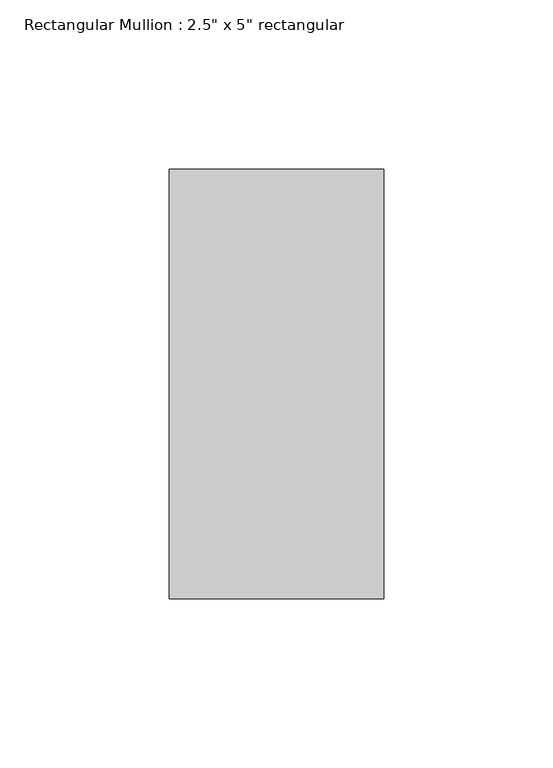
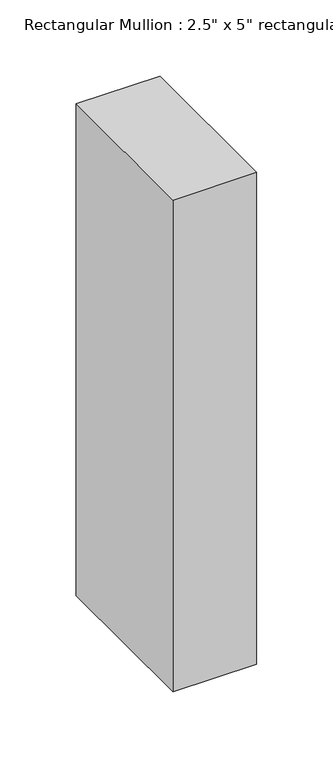
"""IFC4 building model written with IfcOpenShell, lengths in millimetres: member geometry."""

from ifc_helpers import new_model, si_unit, frame, origin, place, context, project, spatial, polyline, outline, extrude, source, transform, mapped, element, save


def member_7096a90e(model_context):
    return source(origin(), model_context, "Body", "SweptSolid", [
        extrude(outline(polyline([(0.0, 63.5), (0.0, -63.5), (-63.5, -63.5), (-63.5, 63.5), (0.0, 63.5)])), frame((0.0, 0.0, -393.7), z_axis=(0.0, 0.0, 1.0), x_axis=(1.0, 0.0, 0.0)), (0.0, 0.0, 1.0), 393.7),
    ])


if __name__ == "__main__":
    model = new_model("IFC4")
    model_context = context("Model", 3, world=origin())
    ifc_project = project(units=[si_unit("LENGTHUNIT", "METRE", prefix="MILLI")], contexts=[model_context])
    site = spatial("IfcSite", under=ifc_project)
    building = spatial("IfcBuilding", under=site)
    placement = place(None, origin())
    member_shape = member_7096a90e(model_context)
    element("IfcMember", 1, ObjectType="Rectangular Mullion : 2.5\" x 5\" rectangular", at=placement, inside=building, context=model_context, shape_type="MappedRepresentation", body=[
        mapped(member_shape, transform((0.0, 0.0, 0.0), x_axis=(1.0, 0.0, 0.0), y_axis=(0.0, 1.0, 0.0), z_axis=(0.0, 0.0, 1.0))),
    ])
    save(model, "model.ifc")

# Revit data of these elements
# Type "Rectangular Mullion : 2.5\" x 5\" rectangular"
#   built-in parameter 1007304 = 0.416667 (stored number, unit not read)
#   built-in parameter 1007301 = 0.104167 (stored number, unit not read)
#   built-in parameter 1007300 = 0.104167 (stored number, unit not read)
# Element 1 (IfcMember, "Rectangular Mullion : 2.5\" x 5\" rectangular")
#   Materials on its faces: "Aluminum"
# Materials
#   "Aluminum": class "Metal", colour RGB 247 247 247, transparency 0, Description = "Aluminum 6061", Cost = 0
